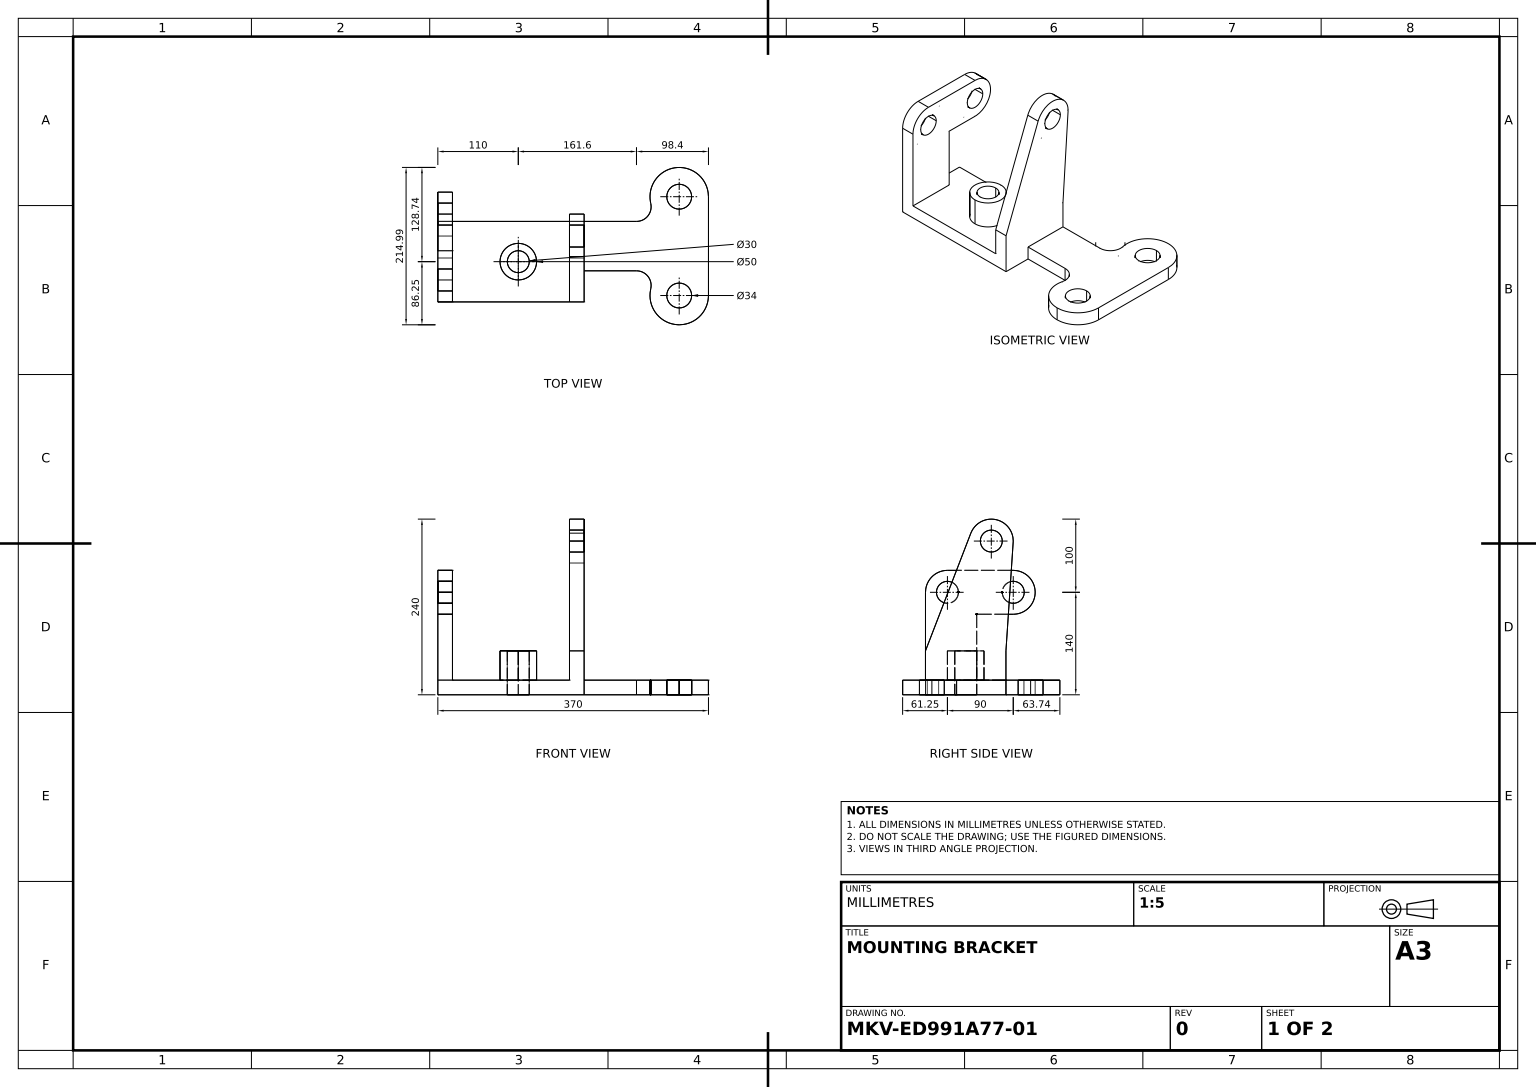
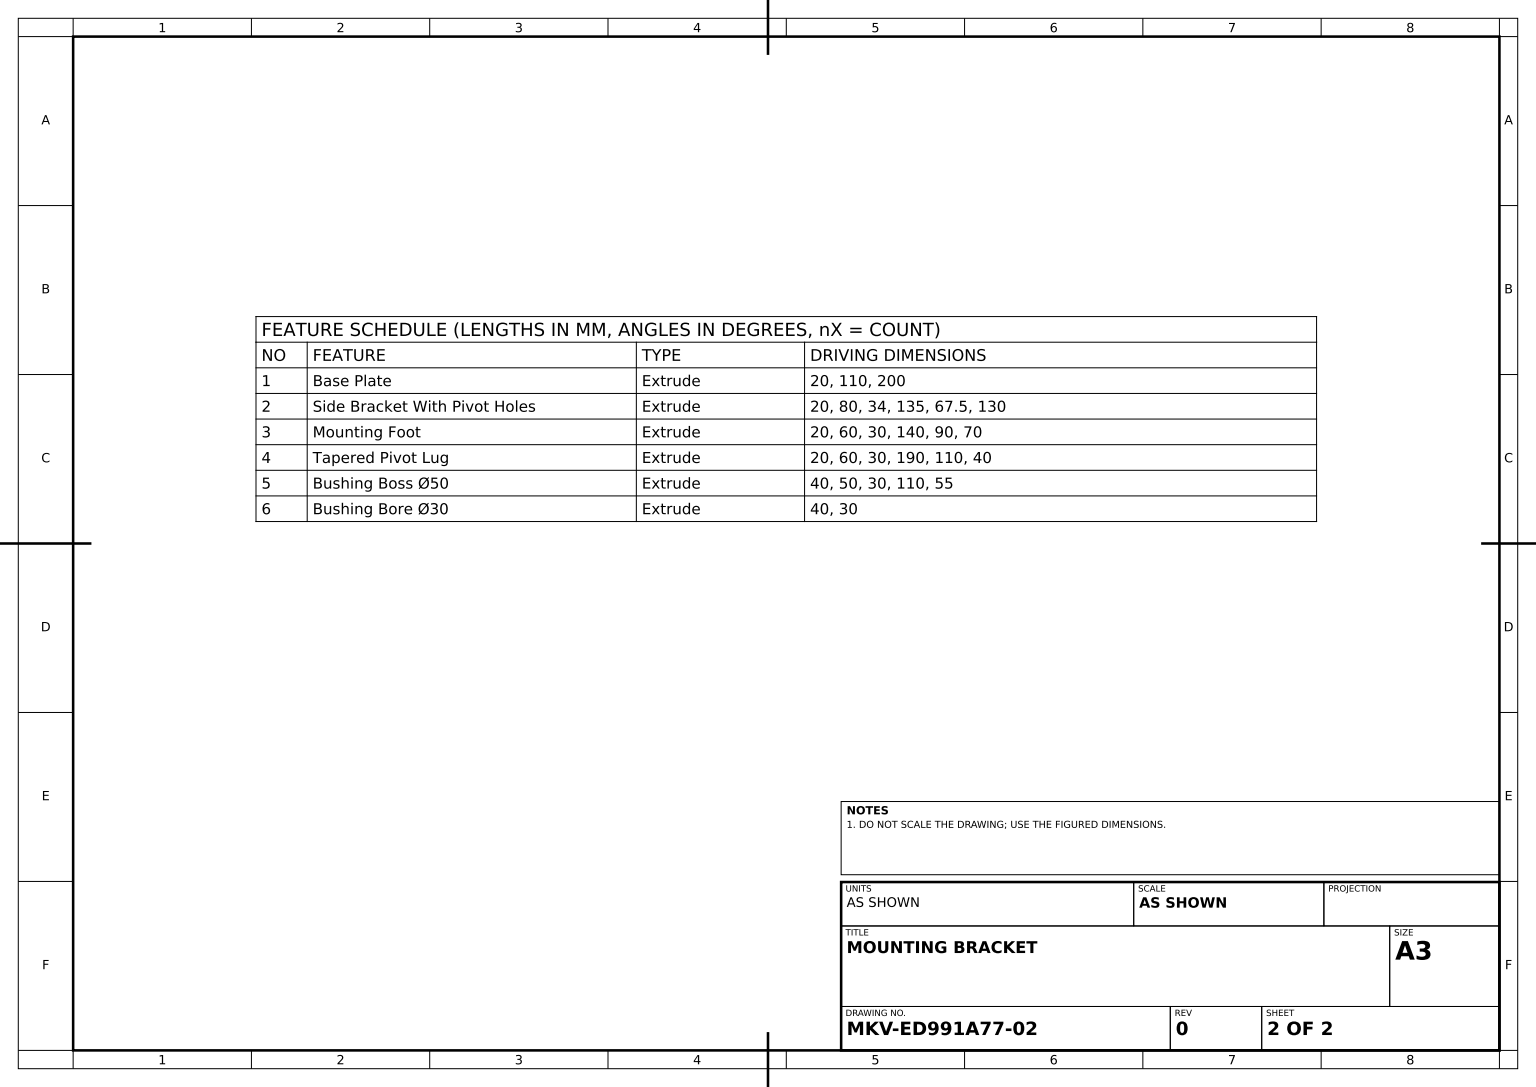
from build123d import *

# Parameters (mm, degrees)
BASE_PLATE_SKETCH_W                 = 200
BASE_PLATE_SKETCH_H                 = 110
BASE_PLATE_DEPTH                    = 20
SIDE_BRACKET_SKETCH_R               = 17
SIDE_BRACKET_WITH_PIVOT_HOLES_DEPTH = 20
MOUNTING_FOOT_SKETCH_R              = 15
MOUNTING_FOOT_SKETCH_W              = 70
MOUNTING_FOOT_SKETCH_H              = 20
MOUNTING_FOOT_DEPTH                 = 20
TAPERED_LUG_SKETCH_R                = 15
TAPERED_PIVOT_LUG_DEPTH             = 20
BUSHING_BOSS_SKETCH_R               = 25
BUSHING_BOSS_SKETCH_R_2             = 15
BUSHING_BOSS_50_DEPTH               = 40
BUSHING_START                       = -40
BUSHING_BORE_SKETCH_R               = 15
BUSHING_BORE_30_DEPTH               = 40


with BuildPart() as part:
    # Base Plate Sketch → Base Plate (new body)
    with BuildSketch(Plane(origin=(0, 0, 0), x_dir=(1, 0, 0), z_dir=(0, 1, 0))):
        Rectangle(BASE_PLATE_SKETCH_W, BASE_PLATE_SKETCH_H)
    extrude(amount=BASE_PLATE_DEPTH)

    # Side Bracket Sketch → Side Bracket With Pivot Holes (add)
    with BuildSketch(Plane(origin=(0, 20, 0), x_dir=(1, 0, 0), z_dir=(0, 1, 0))):
        with BuildLine():
            Line((100, 55), (100, -12.5))
            Line((100, -12.5), (171.596768069, -12.5))
            ThreePointArc((171.596768069, -12.5), (187.275841171, -20.083612979), (191.064512046, -37.083333333))
            ThreePointArc((191.064512046, -37.083333333), (225.385865095, -85.982980748), (270, -46.25))
            Line((270, -46.25), (270, 88.75))
            ThreePointArc((270, 88.75), (225.385865095, 128.482980748), (191.064512046, 79.583333333))
            ThreePointArc((191.064512046, 79.583333333), (187.275841171, 62.583612979), (171.596768069, 55))
            Line((171.596768069, 55), (100, 55))
        make_face()
        with Locations(Location((230, 88.75, 0), (0, 0, 270))):
            Circle(SIDE_BRACKET_SKETCH_R, mode=Mode.SUBTRACT)
        with Locations(Location((230, -46.25, 0), (0, 0, 270))):
            Circle(SIDE_BRACKET_SKETCH_R, mode=Mode.SUBTRACT)
    extrude(amount=-SIDE_BRACKET_WITH_PIVOT_HOLES_DEPTH)

    # Mounting Foot Sketch → Mounting Foot (add)
    # profile 1 of 2: a face of its own
    with BuildSketch(Plane.ZY.offset(100)):
        with BuildLine():
            Line((25, 170), (-65, 170))
            ThreePointArc((-65, 170), (-95, 140), (-65, 110))
            Line((-65, 110), (-15, 110))
            Line((-15, 110), (-15, 20))
            Line((-15, 20), (55, 20))
            Line((55, 20), (55, 140))
            ThreePointArc((55, 140), (46.213203436, 161.213203436), (25, 170))
        make_face()
        with Locations((-65, 140)):
            Circle(MOUNTING_FOOT_SKETCH_R, mode=Mode.SUBTRACT)
        with Locations((25, 140)):
            Circle(MOUNTING_FOOT_SKETCH_R, mode=Mode.SUBTRACT)
    # profile 2 of 2: a face of its own
    with BuildSketch(Plane.ZY.offset(100)):
        with Locations((20, 10)):
            Rectangle(MOUNTING_FOOT_SKETCH_W, MOUNTING_FOOT_SKETCH_H)
    extrude(amount=-MOUNTING_FOOT_DEPTH)

    # Tapered Lug Sketch → Tapered Pivot Lug (add)
    with BuildSketch(Plane(origin=(100, 0, 0), x_dir=(0, 0, -1), z_dir=(1, 0, 0))):
        with BuildLine():
            Line((-55, 60), (-55, 20))
            Line((-55, 20), (-12.5, 20))
            Line((-12.5, 20), (55, 20))
            Line((55, 20), (55, 60))
            Line((55, 60), (64.734513274, 206.017699115))
            Line((64.734513274, 206.017699115), (65, 210))
            ThreePointArc((65, 210), (40.489921368, 239.493402031), (7.009282442, 220.794430535))
            Line((7.009282442, 220.794430535), (-55, 60))
        make_face()
        with Locations((35, 210)):
            Circle(TAPERED_LUG_SKETCH_R, mode=Mode.SUBTRACT)
    extrude(amount=-TAPERED_PIVOT_LUG_DEPTH)

    # Bushing Boss Sketch → Bushing Boss Ø50 (add)
    with BuildSketch(Plane(origin=(0, 20, 0), x_dir=(1, 0, 0), z_dir=(0, 1, 0))):
        with Locations(Location((10, 0, 0), (0, 0, 270))):
            Circle(BUSHING_BOSS_SKETCH_R)
        with Locations(Location((10, 0, 0), (0, 0, 270))):
            Circle(BUSHING_BOSS_SKETCH_R_2, mode=Mode.SUBTRACT)
    extrude(amount=BUSHING_BOSS_50_DEPTH)

    # Bushing Bore Sketch → Bushing Bore Ø30 (cut)
    with BuildSketch(Plane(origin=(0, 20, 0), x_dir=(1, 0, 0), z_dir=(0, 1, 0)).offset(BUSHING_START)):
        with Locations(Location((10, 0, 0), (0, 0, 270))):
            Circle(BUSHING_BORE_SKETCH_R)
    extrude(amount=BUSHING_BORE_30_DEPTH, mode=Mode.SUBTRACT)


solid = part.part
